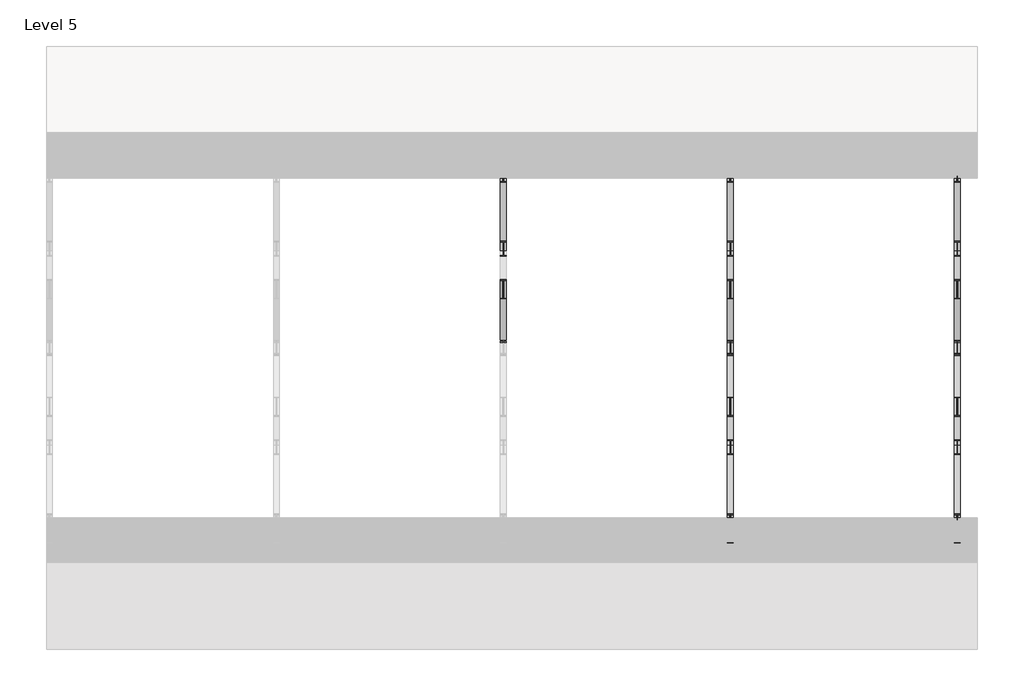
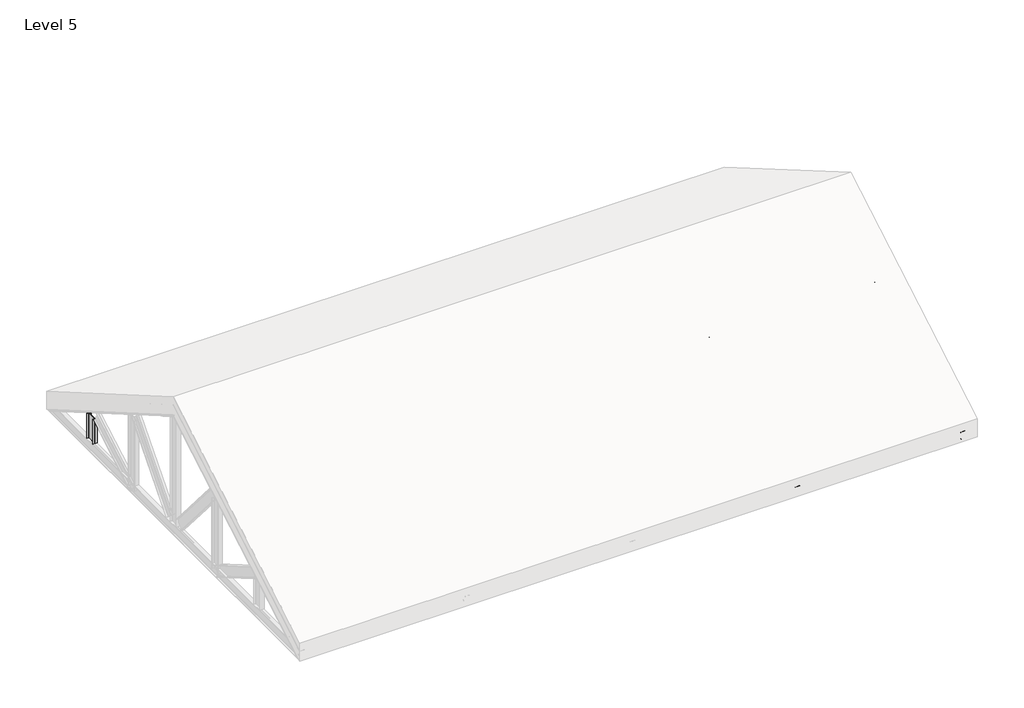
# One storey, part 2 of 2: 31 beams.
"""IFC4 building model written with IfcOpenShell, lengths in millimetres."""

from ifc_helpers import new_model, si_unit, frame, origin, place, context, project, spatial, polyline, circle_curve, ellipse_curve, transform, mapped, element, save
from ifc_brep_helpers import plane_surface, revolved_surface, advanced_brep
from components import ub_universal_beams_ub254x102x28_e74905dc, ub_universal_beams_ub254x102x28_1dca85a9, ub_universal_beams_ub254x102x28_3582687b, ub_universal_beams_ub254x102x28_9eef3cd1, ub_universal_beams_ub254x102x28_f7ef6108, ub_universal_beams_ub254x102x28_93a23aa5, ub_universal_beams_ub254x102x28_1ec9d6d8, ub_universal_beams_ub254x102x28_a06fb1b7

model = new_model("IFC4")

# Units and contexts
model_context = context("Model", 3, world=origin())
ifc_project = project(units=[si_unit("LENGTHUNIT", "METRE", prefix="MILLI")], contexts=[model_context])

# Site, building, storey
site = spatial("IfcSite", under=ifc_project)
building = spatial("IfcBuilding", under=site)
storey = spatial("IfcBuildingStorey", under=building, Name="Level 5", Elevation=9144.0)

# Beams
placement = place(None, origin())
element("IfcBeam", 1, ObjectType="UB-Universal Beams : UB254x102x28", at=placement, inside=storey, context=model_context, shape_type="AdvancedBrep", body=[
    advanced_brep(
    [(-879.5620752, 9795.4298445, 9040.0618528), (-879.5620752, 9790.4089662, 9031.4136864), (-981.7620752, 9790.4089662, 9031.4136864), (-981.7620752, 9795.4298445, 9040.0618528), (-941.4120752, 9795.4298445, 9040.0618528), (-933.8120752, 9799.245712, 9046.6344592), (-933.8120752, 9912.3158911, 9241.3911653), (-941.4120752, 9916.1317586, 9247.9637718), (-981.7620752, 9916.1317586, 9247.9637718), (-981.7620752, 9921.1526369, 9256.6119381), (-879.5620752, 9921.1526369, 9256.6119381), (-879.5620752, 9916.1317586, 9247.9637718), (-919.9120752, 9916.1317586, 9247.9637718), (-927.5120752, 9912.3158911, 9241.3911653), (-927.5120752, 9799.245712, 9046.6344592), (-919.9120752, 9795.4298445, 9040.0618528), (-919.9120752, 4605.8028699, 12053.0109991), (-879.5620752, 4605.8028699, 12053.0109991), (-927.5120752, 4605.8028699, 12061.7989892), (-927.5120752, 4605.8028699, 12322.2010108), (-919.9120752, 4605.8028699, 12330.9890009), (-879.5620752, 4605.8028699, 12330.9890009), (-879.5620752, 4605.8028699, 12342.5521457), (-981.7620752, 4605.8028699, 12342.5521457), (-981.7620752, 4605.8028699, 12330.9890009), (-941.4120752, 4605.8028699, 12330.9890009), (-933.8120752, 4605.8028699, 12322.2010108), (-933.8120752, 4605.8028699, 12061.7989892), (-941.4120752, 4605.8028699, 12053.0109991), (-981.7620752, 4605.8028699, 12053.0109991), (-981.7620752, 4605.8028699, 12041.4478543), (-879.5620752, 4605.8028699, 12041.4478543)],
    [
        (0, 1),
        (1, 2),
        (2, 3),
        (3, 4),
        (4, 5, circle_curve(frame((-941.4120752, 9799.245712, 9046.6344592), z_axis=(0.0, -0.8648166348106393, 0.5020878291243489), x_axis=(-1.0, 0.0, 0.0)), 7.6)),
        (5, 6),
        (6, 7, circle_curve(frame((-941.4120752, 9912.3158911, 9241.3911653), z_axis=(0.0, -0.8648166348106393, 0.5020878291243489), x_axis=(-1.0, 0.0, 0.0)), 7.6)),
        (7, 8),
        (8, 9),
        (9, 10),
        (10, 11),
        (11, 12),
        (12, 13, circle_curve(frame((-919.9120752, 9912.3158911, 9241.3911653), z_axis=(0.0, -0.8648166348106393, 0.5020878291243489), x_axis=(-1.0, 0.0, 0.0)), 7.6)),
        (13, 14),
        (14, 15, circle_curve(frame((-919.9120752, 9799.245712, 9046.6344592), z_axis=(0.0, -0.8648166348106393, 0.5020878291243489), x_axis=(-1.0, 0.0, 0.0)), 7.6)),
        (15, 0),
        (16, 17),
        (17, 0),
        (15, 16),
        (18, 16, ellipse_curve(frame((-919.9120752, 4605.8028699, 12061.7989892), z_axis=(0.0, -1.0, 0.0), x_axis=(0.0, 0.0, -1.0)), 8.7879901, 7.6)),
        (14, 18),
        (19, 18),
        (13, 19),
        (20, 19, ellipse_curve(frame((-919.9120752, 4605.8028699, 12322.2010108), z_axis=(0.0, -1.0, 0.0), x_axis=(0.0, 0.0, -1.0)), 8.7879901, 7.6)),
        (12, 20),
        (21, 20),
        (11, 21),
        (22, 21),
        (10, 22),
        (23, 22),
        (9, 23),
        (24, 23),
        (8, 24),
        (25, 24),
        (7, 25),
        (26, 25, ellipse_curve(frame((-941.4120752, 4605.8028699, 12322.2010108), z_axis=(0.0, -1.0, 0.0), x_axis=(0.0, 0.0, -1.0)), 8.7879901, 7.6)),
        (6, 26),
        (27, 26),
        (5, 27),
        (28, 27, ellipse_curve(frame((-941.4120752, 4605.8028699, 12061.7989892), z_axis=(0.0, -1.0, 0.0), x_axis=(0.0, 0.0, -1.0)), 8.7879901, 7.6)),
        (4, 28),
        (29, 28),
        (3, 29),
        (30, 29),
        (2, 30),
        (31, 30),
        (1, 31),
        (17, 31),
    ],
    [
        plane_surface(frame((-930.6620752, 9855.7808016, 9144.0128123), z_axis=(0.0, 0.8648166348106393, -0.5020878291243489), x_axis=(0.0, 0.5020878291243489, 0.8648166348106393))),
        plane_surface(frame((-879.5620752, 4545.4739812, 12088.0362282), z_axis=(0.0, 0.5020878291243489, 0.8648166348106393), x_axis=(0.0, 0.8648166348106393, -0.5020878291243489))),
        revolved_surface(polyline([(-927.5120752, 9799.245712003027, 9046.634459205212), (-927.5120752, 4601.987002407376, 12064.01437289046)]), (-919.9120752, 4549.2898487, 12094.6088347), (0.0, 0.8648166348106393, -0.5020878291243489)),
        plane_surface(frame((-927.5120752, 4549.2898487, 12094.6088347), z_axis=(1.0, 0.0, 0.0), x_axis=(0.0, 0.8648166348106393, -0.5020878291243489))),
        revolved_surface(polyline([(-927.5120752, 9912.315891103026, 9241.391165305211), (-927.5120752, 4601.987002367825, 12324.416394422336)]), (-919.9120752, 4662.3600278, 12289.3655408), (0.0, 0.8648166348106393, -0.5020878291243489)),
        plane_surface(frame((-919.9120752, 4666.1758953, 12295.9381472), z_axis=(0.0, -0.5020878291243489, -0.8648166348106393), x_axis=(0.0, 0.8648166348106393, -0.5020878291243489))),
        plane_surface(frame((-879.5620752, 4666.1758953, 12295.9381472), z_axis=(1.0, 0.0, 0.0), x_axis=(0.0, 0.8648166348106393, -0.5020878291243489))),
        plane_surface(frame((-879.5620752, 4671.1967736, 12304.5863136), z_axis=(0.0, 0.5020878291243489, 0.8648166348106393), x_axis=(0.0, 0.8648166348106393, -0.5020878291243489))),
        plane_surface(frame((-981.7620752, 4671.1967736, 12304.5863136), z_axis=(-1.0, 0.0, 0.0), x_axis=(0.0, 0.8648166348106393, -0.5020878291243489))),
        plane_surface(frame((-981.7620752, 4666.1758953, 12295.9381472), z_axis=(0.0, -0.5020878291243489, -0.8648166348106393), x_axis=(0.0, 0.8648166348106393, -0.5020878291243489))),
        revolved_surface(polyline([(-949.0120752, 9912.315891103026, 9241.391165305211), (-949.0120752, 4601.987002367825, 12324.416394422336)]), (-941.4120752, 4662.3600278, 12289.3655408), (0.0, 0.8648166348106393, -0.5020878291243489)),
        plane_surface(frame((-933.8120752, 4662.3600278, 12289.3655408), z_axis=(-1.0, 0.0, 0.0), x_axis=(0.0, 0.8648166348106393, -0.5020878291243489))),
        revolved_surface(polyline([(-949.0120752, 9799.245712003027, 9046.634459205212), (-949.0120752, 4601.987002407376, 12064.01437289046)]), (-941.4120752, 4549.2898487, 12094.6088347), (0.0, 0.8648166348106393, -0.5020878291243489)),
        plane_surface(frame((-941.4120752, 4545.4739812, 12088.0362282), z_axis=(0.0, 0.5020878291243489, 0.8648166348106393), x_axis=(0.0, 0.8648166348106393, -0.5020878291243489))),
        plane_surface(frame((-981.7620752, 4545.4739812, 12088.0362282), z_axis=(-1.0, 0.0, 0.0), x_axis=(0.0, 0.8648166348106393, -0.5020878291243489))),
        plane_surface(frame((-981.7620752, 4540.4531029, 12079.3880619), z_axis=(0.0, -0.5020878291243489, -0.8648166348106393), x_axis=(0.0, 0.8648166348106393, -0.5020878291243489))),
        plane_surface(frame((-879.5620752, 4540.4531029, 12079.3880619), z_axis=(1.0, 0.0, 0.0), x_axis=(0.0, 0.8648166348106393, -0.5020878291243489))),
        plane_surface(frame((-930.6620752, 4605.8028699, 12342.5521457), z_axis=(0.0, -1.0, 0.0), x_axis=(0.0, 0.0, 1.0))),
    ],
    [
        (0, [[1, 2, 3, 4, 5, 6, 7, 8, 9, 10, 11, 12, 13, 14, 15, 16]]),
        (1, [[17, 18, -16, 19]]),
        (2, [[20, -19, -15, 21]]),
        (3, [[22, -21, -14, 23]]),
        (4, [[24, -23, -13, 25]]),
        (5, [[26, -25, -12, 27]]),
        (6, [[28, -27, -11, 29]]),
        (7, [[30, -29, -10, 31]]),
        (8, [[32, -31, -9, 33]]),
        (9, [[34, -33, -8, 35]]),
        (10, [[36, -35, -7, 37]]),
        (11, [[38, -37, -6, 39]]),
        (12, [[40, -39, -5, 41]]),
        (13, [[42, -41, -4, 43]]),
        (14, [[44, -43, -3, 45]]),
        (15, [[46, -45, -2, 47]]),
        (16, [[48, -47, -1, -18]]),
        (17, [[-17, -20, -22, -24, -26, -28, -30, -32, -34, -36, -38, -40, -42, -44, -46, -48]]),
    ],
),
])
element("IfcBeam", 2, ObjectType="UB-Universal Beams : UB254x102x28", at=placement, inside=storey, context=model_context, shape_type="AdvancedBrep", body=[
    advanced_brep(
    [(3120.4379248, 9795.4298445, 9040.0618528), (3120.4379248, 9790.4089662, 9031.4136864), (3018.2379248, 9790.4089662, 9031.4136864), (3018.2379248, 9795.4298445, 9040.0618528), (3058.5879248, 9795.4298445, 9040.0618528), (3066.1879248, 9799.245712, 9046.6344592), (3066.1879248, 9912.3158911, 9241.3911653), (3058.5879248, 9916.1317586, 9247.9637718), (3018.2379248, 9916.1317586, 9247.9637718), (3018.2379248, 9921.1526369, 9256.6119381), (3120.4379248, 9921.1526369, 9256.6119381), (3120.4379248, 9916.1317586, 9247.9637718), (3080.0879248, 9916.1317586, 9247.9637718), (3072.4879248, 9912.3158911, 9241.3911653), (3072.4879248, 9799.245712, 9046.6344592), (3080.0879248, 9795.4298445, 9040.0618528), (3080.0879248, 4605.8028699, 12053.0109991), (3120.4379248, 4605.8028699, 12053.0109991), (3072.4879248, 4605.8028699, 12061.7989892), (3072.4879248, 4605.8028699, 12322.2010108), (3080.0879248, 4605.8028699, 12330.9890009), (3120.4379248, 4605.8028699, 12330.9890009), (3120.4379248, 4605.8028699, 12342.5521457), (3018.2379248, 4605.8028699, 12342.5521457), (3018.2379248, 4605.8028699, 12330.9890009), (3058.5879248, 4605.8028699, 12330.9890009), (3066.1879248, 4605.8028699, 12322.2010108), (3066.1879248, 4605.8028699, 12061.7989892), (3058.5879248, 4605.8028699, 12053.0109991), (3018.2379248, 4605.8028699, 12053.0109991), (3018.2379248, 4605.8028699, 12041.4478543), (3120.4379248, 4605.8028699, 12041.4478543)],
    [
        (0, 1),
        (1, 2),
        (2, 3),
        (3, 4),
        (4, 5, circle_curve(frame((3058.5879248, 9799.245712, 9046.6344592), z_axis=(0.0, -0.8648166348106393, 0.5020878291243489), x_axis=(-1.0, 0.0, 0.0)), 7.6)),
        (5, 6),
        (6, 7, circle_curve(frame((3058.5879248, 9912.3158911, 9241.3911653), z_axis=(0.0, -0.8648166348106393, 0.5020878291243489), x_axis=(-1.0, 0.0, 0.0)), 7.6)),
        (7, 8),
        (8, 9),
        (9, 10),
        (10, 11),
        (11, 12),
        (12, 13, circle_curve(frame((3080.0879248, 9912.3158911, 9241.3911653), z_axis=(0.0, -0.8648166348106393, 0.5020878291243489), x_axis=(-1.0, 0.0, 0.0)), 7.6)),
        (13, 14),
        (14, 15, circle_curve(frame((3080.0879248, 9799.245712, 9046.6344592), z_axis=(0.0, -0.8648166348106393, 0.5020878291243489), x_axis=(-1.0, 0.0, 0.0)), 7.6)),
        (15, 0),
        (16, 17),
        (17, 0),
        (15, 16),
        (18, 16, ellipse_curve(frame((3080.0879248, 4605.8028699, 12061.7989892), z_axis=(0.0, -1.0, 0.0), x_axis=(0.0, 0.0, -1.0)), 8.7879901, 7.6)),
        (14, 18),
        (19, 18),
        (13, 19),
        (20, 19, ellipse_curve(frame((3080.0879248, 4605.8028699, 12322.2010108), z_axis=(0.0, -1.0, 0.0), x_axis=(0.0, 0.0, -1.0)), 8.7879901, 7.6)),
        (12, 20),
        (21, 20),
        (11, 21),
        (22, 21),
        (10, 22),
        (23, 22),
        (9, 23),
        (24, 23),
        (8, 24),
        (25, 24),
        (7, 25),
        (26, 25, ellipse_curve(frame((3058.5879248, 4605.8028699, 12322.2010108), z_axis=(0.0, -1.0, 0.0), x_axis=(0.0, 0.0, -1.0)), 8.7879901, 7.6)),
        (6, 26),
        (27, 26),
        (5, 27),
        (28, 27, ellipse_curve(frame((3058.5879248, 4605.8028699, 12061.7989892), z_axis=(0.0, -1.0, 0.0), x_axis=(0.0, 0.0, -1.0)), 8.7879901, 7.6)),
        (4, 28),
        (29, 28),
        (3, 29),
        (30, 29),
        (2, 30),
        (31, 30),
        (1, 31),
        (17, 31),
    ],
    [
        plane_surface(frame((3069.3379248, 9855.7808016, 9144.0128123), z_axis=(0.0, 0.8648166348106393, -0.5020878291243489), x_axis=(0.0, 0.5020878291243489, 0.8648166348106393))),
        plane_surface(frame((3120.4379248, 4545.4739812, 12088.0362282), z_axis=(0.0, 0.5020878291243489, 0.8648166348106393), x_axis=(0.0, 0.8648166348106393, -0.5020878291243489))),
        revolved_surface(polyline([(3072.4879248, 9799.245712003027, 9046.634459205212), (3072.4879248, 4601.987002407376, 12064.01437289046)]), (3080.0879248, 4549.2898487, 12094.6088347), (0.0, 0.8648166348106393, -0.5020878291243489)),
        plane_surface(frame((3072.4879248, 4549.2898487, 12094.6088347), z_axis=(1.0, 0.0, 0.0), x_axis=(0.0, 0.8648166348106393, -0.5020878291243489))),
        revolved_surface(polyline([(3072.4879248, 9912.315891103026, 9241.391165305211), (3072.4879248, 4601.987002367825, 12324.416394422336)]), (3080.0879248, 4662.3600278, 12289.3655408), (0.0, 0.8648166348106393, -0.5020878291243489)),
        plane_surface(frame((3080.0879248, 4666.1758953, 12295.9381472), z_axis=(0.0, -0.5020878291243489, -0.8648166348106393), x_axis=(0.0, 0.8648166348106393, -0.5020878291243489))),
        plane_surface(frame((3120.4379248, 4666.1758953, 12295.9381472), z_axis=(1.0, 0.0, 0.0), x_axis=(0.0, 0.8648166348106393, -0.5020878291243489))),
        plane_surface(frame((3120.4379248, 4671.1967736, 12304.5863136), z_axis=(0.0, 0.5020878291243489, 0.8648166348106393), x_axis=(0.0, 0.8648166348106393, -0.5020878291243489))),
        plane_surface(frame((3018.2379248, 4671.1967736, 12304.5863136), z_axis=(-1.0, 0.0, 0.0), x_axis=(0.0, 0.8648166348106393, -0.5020878291243489))),
        plane_surface(frame((3018.2379248, 4666.1758953, 12295.9381472), z_axis=(0.0, -0.5020878291243489, -0.8648166348106393), x_axis=(0.0, 0.8648166348106393, -0.5020878291243489))),
        revolved_surface(polyline([(3050.9879248, 9912.315891103026, 9241.391165305211), (3050.9879248, 4601.987002367825, 12324.416394422336)]), (3058.5879248, 4662.3600278, 12289.3655408), (0.0, 0.8648166348106393, -0.5020878291243489)),
        plane_surface(frame((3066.1879248, 4662.3600278, 12289.3655408), z_axis=(-1.0, 0.0, 0.0), x_axis=(0.0, 0.8648166348106393, -0.5020878291243489))),
        revolved_surface(polyline([(3050.9879248, 9799.245712003027, 9046.634459205212), (3050.9879248, 4601.987002407376, 12064.01437289046)]), (3058.5879248, 4549.2898487, 12094.6088347), (0.0, 0.8648166348106393, -0.5020878291243489)),
        plane_surface(frame((3058.5879248, 4545.4739812, 12088.0362282), z_axis=(0.0, 0.5020878291243489, 0.8648166348106393), x_axis=(0.0, 0.8648166348106393, -0.5020878291243489))),
        plane_surface(frame((3018.2379248, 4545.4739812, 12088.0362282), z_axis=(-1.0, 0.0, 0.0), x_axis=(0.0, 0.8648166348106393, -0.5020878291243489))),
        plane_surface(frame((3018.2379248, 4540.4531029, 12079.3880619), z_axis=(0.0, -0.5020878291243489, -0.8648166348106393), x_axis=(0.0, 0.8648166348106393, -0.5020878291243489))),
        plane_surface(frame((3120.4379248, 4540.4531029, 12079.3880619), z_axis=(1.0, 0.0, 0.0), x_axis=(0.0, 0.8648166348106393, -0.5020878291243489))),
        plane_surface(frame((3069.3379248, 4605.8028699, 12342.5521457), z_axis=(0.0, -1.0, 0.0), x_axis=(0.0, 0.0, 1.0))),
    ],
    [
        (0, [[1, 2, 3, 4, 5, 6, 7, 8, 9, 10, 11, 12, 13, 14, 15, 16]]),
        (1, [[17, 18, -16, 19]]),
        (2, [[20, -19, -15, 21]]),
        (3, [[22, -21, -14, 23]]),
        (4, [[24, -23, -13, 25]]),
        (5, [[26, -25, -12, 27]]),
        (6, [[28, -27, -11, 29]]),
        (7, [[30, -29, -10, 31]]),
        (8, [[32, -31, -9, 33]]),
        (9, [[34, -33, -8, 35]]),
        (10, [[36, -35, -7, 37]]),
        (11, [[38, -37, -6, 39]]),
        (12, [[40, -39, -5, 41]]),
        (13, [[42, -41, -4, 43]]),
        (14, [[44, -43, -3, 45]]),
        (15, [[46, -45, -2, 47]]),
        (16, [[48, -47, -1, -18]]),
        (17, [[-17, -20, -22, -24, -26, -28, -30, -32, -34, -36, -38, -40, -42, -44, -46, -48]]),
    ],
),
])
element("IfcBeam", 3, ObjectType="UB-Universal Beams : UB254x102x28", at=placement, inside=storey, context=model_context, shape_type="AdvancedBrep", body=[
    advanced_brep(
    [(3120.4379248, -583.8241047, 9040.0618528), (3080.0879248, -583.8241047, 9040.0618528), (3072.4879248, -587.6399722, 9046.6344592), (3072.4879248, -700.7101513, 9241.3911653), (3080.0879248, -704.5260188, 9247.9637718), (3120.4379248, -704.5260188, 9247.9637718), (3120.4379248, -709.5468971, 9256.6119381), (3018.2379248, -709.5468971, 9256.6119381), (3018.2379248, -704.5260188, 9247.9637718), (3058.5879248, -704.5260188, 9247.9637718), (3066.1879248, -700.7101513, 9241.3911653), (3066.1879248, -587.6399722, 9046.6344592), (3058.5879248, -583.8241047, 9040.0618528), (3018.2379248, -583.8241047, 9040.0618528), (3018.2379248, -578.8032264, 9031.4136864), (3120.4379248, -578.8032264, 9031.4136864), (3120.4379248, 4605.8028699, 12053.0109991), (3080.0879248, 4605.8028699, 12053.0109991), (3072.4879248, 4605.8028699, 12061.7989892), (3072.4879248, 4605.8028699, 12322.2010108), (3080.0879248, 4605.8028699, 12330.9890009), (3120.4379248, 4605.8028699, 12330.9890009), (3120.4379248, 4605.8028699, 12342.5521457), (3018.2379248, 4605.8028699, 12342.5521457), (3018.2379248, 4605.8028699, 12330.9890009), (3058.5879248, 4605.8028699, 12330.9890009), (3066.1879248, 4605.8028699, 12322.2010108), (3066.1879248, 4605.8028699, 12061.7989892), (3058.5879248, 4605.8028699, 12053.0109991), (3018.2379248, 4605.8028699, 12053.0109991), (3018.2379248, 4605.8028699, 12041.4478543), (3120.4379248, 4605.8028699, 12041.4478543)],
    [
        (0, 1),
        (1, 2, circle_curve(frame((3080.0879248, -587.6399722, 9046.6344592), z_axis=(0.0, 0.8648166348106395, 0.5020878291243485), x_axis=(-1.0, 0.0, 0.0)), 7.6)),
        (2, 3),
        (3, 4, circle_curve(frame((3080.0879248, -700.7101513, 9241.3911653), z_axis=(0.0, 0.8648166348106395, 0.5020878291243485), x_axis=(-1.0, 0.0, 0.0)), 7.6)),
        (4, 5),
        (5, 6),
        (6, 7),
        (7, 8),
        (8, 9),
        (9, 10, circle_curve(frame((3058.5879248, -700.7101513, 9241.3911653), z_axis=(0.0, 0.8648166348106395, 0.5020878291243485), x_axis=(-1.0, 0.0, 0.0)), 7.6)),
        (10, 11),
        (11, 12, circle_curve(frame((3058.5879248, -587.6399722, 9046.6344592), z_axis=(0.0, 0.8648166348106395, 0.5020878291243485), x_axis=(-1.0, 0.0, 0.0)), 7.6)),
        (12, 13),
        (13, 14),
        (14, 15),
        (15, 0),
        (0, 16),
        (16, 17),
        (17, 1),
        (17, 18, ellipse_curve(frame((3080.0879248, 4605.8028699, 12061.7989892), z_axis=(0.0, 1.0, 0.0), x_axis=(0.0, 0.0, 1.0)), 8.7879901, 7.6)),
        (18, 2),
        (18, 19),
        (19, 3),
        (19, 20, ellipse_curve(frame((3080.0879248, 4605.8028699, 12322.2010108), z_axis=(0.0, 1.0, 0.0), x_axis=(0.0, 0.0, 1.0)), 8.7879901, 7.6)),
        (20, 4),
        (20, 21),
        (21, 5),
        (21, 22),
        (22, 6),
        (22, 23),
        (23, 7),
        (23, 24),
        (24, 8),
        (24, 25),
        (25, 9),
        (25, 26, ellipse_curve(frame((3058.5879248, 4605.8028699, 12322.2010108), z_axis=(0.0, 1.0, 0.0), x_axis=(0.0, 0.0, 1.0)), 8.7879901, 7.6)),
        (26, 10),
        (26, 27),
        (27, 11),
        (27, 28, ellipse_curve(frame((3058.5879248, 4605.8028699, 12061.7989892), z_axis=(0.0, 1.0, 0.0), x_axis=(0.0, 0.0, 1.0)), 8.7879901, 7.6)),
        (28, 12),
        (28, 29),
        (29, 13),
        (29, 30),
        (30, 14),
        (30, 31),
        (31, 15),
        (31, 16),
    ],
    [
        plane_surface(frame((3069.3379248, -644.1750617, 9144.0128123), z_axis=(0.0, -0.8648166348106395, -0.5020878291243485), x_axis=(0.0, -0.5020878291243485, 0.8648166348106395))),
        plane_surface(frame((3120.4379248, -583.8241047, 9040.0618528), z_axis=(0.0, -0.5020878291243485, 0.8648166348106395), x_axis=(0.0, 0.8648166348106395, 0.5020878291243485))),
        revolved_surface(polyline([(3072.4879248, 4609.618737395652, 12064.014372885247), (3072.4879248, -587.6399722, 9046.6344592)]), (3080.0879248, -587.6399722, 9046.6344592), (0.0, 0.8648166348106395, 0.5020878291243485)),
        plane_surface(frame((3072.4879248, -587.6399722, 9046.6344592), z_axis=(1.0, 0.0, 0.0), x_axis=(0.0, 0.8648166348106395, 0.5020878291243485))),
        revolved_surface(polyline([(3072.4879248, 4609.618737435201, 12324.416394417123), (3072.4879248, -700.7101513, 9241.3911653)]), (3080.0879248, -700.7101513, 9241.3911653), (0.0, 0.8648166348106395, 0.5020878291243485)),
        plane_surface(frame((3080.0879248, -704.5260188, 9247.9637718), z_axis=(0.0, 0.5020878291243485, -0.8648166348106395), x_axis=(0.0, 0.8648166348106395, 0.5020878291243485))),
        plane_surface(frame((3120.4379248, -704.5260188, 9247.9637718), z_axis=(1.0, 0.0, 0.0), x_axis=(0.0, 0.8648166348106395, 0.5020878291243485))),
        plane_surface(frame((3120.4379248, -709.5468971, 9256.6119381), z_axis=(0.0, -0.5020878291243485, 0.8648166348106395), x_axis=(0.0, 0.8648166348106395, 0.5020878291243485))),
        plane_surface(frame((3018.2379248, -709.5468971, 9256.6119381), z_axis=(-1.0, 0.0, 0.0), x_axis=(0.0, 0.8648166348106395, 0.5020878291243485))),
        plane_surface(frame((3018.2379248, -704.5260188, 9247.9637718), z_axis=(0.0, 0.5020878291243485, -0.8648166348106395), x_axis=(0.0, 0.8648166348106395, 0.5020878291243485))),
        revolved_surface(polyline([(3050.9879248, 4609.618737435201, 12324.416394417123), (3050.9879248, -700.7101513, 9241.3911653)]), (3058.5879248, -700.7101513, 9241.3911653), (0.0, 0.8648166348106395, 0.5020878291243485)),
        plane_surface(frame((3066.1879248, -700.7101513, 9241.3911653), z_axis=(-1.0, 0.0, 0.0), x_axis=(0.0, 0.8648166348106395, 0.5020878291243485))),
        revolved_surface(polyline([(3050.9879248, 4609.618737395652, 12064.014372885247), (3050.9879248, -587.6399722, 9046.6344592)]), (3058.5879248, -587.6399722, 9046.6344592), (0.0, 0.8648166348106395, 0.5020878291243485)),
        plane_surface(frame((3058.5879248, -583.8241047, 9040.0618528), z_axis=(0.0, -0.5020878291243485, 0.8648166348106395), x_axis=(0.0, 0.8648166348106395, 0.5020878291243485))),
        plane_surface(frame((3018.2379248, -583.8241047, 9040.0618528), z_axis=(-1.0, 0.0, 0.0), x_axis=(0.0, 0.8648166348106395, 0.5020878291243485))),
        plane_surface(frame((3018.2379248, -578.8032264, 9031.4136864), z_axis=(0.0, 0.5020878291243485, -0.8648166348106395), x_axis=(0.0, 0.8648166348106395, 0.5020878291243485))),
        plane_surface(frame((3120.4379248, -578.8032264, 9031.4136864), z_axis=(1.0, 0.0, 0.0), x_axis=(0.0, 0.8648166348106395, 0.5020878291243485))),
        plane_surface(frame((3069.3379248, 4605.8028699, 12342.5521457), z_axis=(0.0, 1.0, 0.0), x_axis=(0.0, 0.0, -1.0))),
    ],
    [
        (0, [[1, 2, 3, 4, 5, 6, 7, 8, 9, 10, 11, 12, 13, 14, 15, 16]]),
        (1, [[-1, 17, 18, 19]]),
        (2, [[-2, -19, 20, 21]]),
        (3, [[-3, -21, 22, 23]]),
        (4, [[-4, -23, 24, 25]]),
        (5, [[-5, -25, 26, 27]]),
        (6, [[-6, -27, 28, 29]]),
        (7, [[-7, -29, 30, 31]]),
        (8, [[-8, -31, 32, 33]]),
        (9, [[-9, -33, 34, 35]]),
        (10, [[-10, -35, 36, 37]]),
        (11, [[-11, -37, 38, 39]]),
        (12, [[-12, -39, 40, 41]]),
        (13, [[-13, -41, 42, 43]]),
        (14, [[-14, -43, 44, 45]]),
        (15, [[-15, -45, 46, 47]]),
        (16, [[-16, -47, 48, -17]]),
        (17, [[-48, -46, -44, -42, -40, -38, -36, -34, -32, -30, -28, -26, -24, -22, -20, -18]]),
    ],
),
])
element("IfcBeam", 4, ObjectType="UB-Universal Beams : UB254x102x28", at=placement, inside=storey, context=model_context, shape_type="AdvancedBrep", body=[
    advanced_brep(
    [(7120.4379248, 9795.4298445, 9040.0618528), (7120.4379248, 9790.4089662, 9031.4136864), (7018.2379248, 9790.4089662, 9031.4136864), (7018.2379248, 9795.4298445, 9040.0618528), (7058.5879248, 9795.4298445, 9040.0618528), (7066.1879248, 9799.245712, 9046.6344592), (7066.1879248, 9912.3158911, 9241.3911653), (7058.5879248, 9916.1317586, 9247.9637718), (7018.2379248, 9916.1317586, 9247.9637718), (7018.2379248, 9921.1526369, 9256.6119381), (7120.4379248, 9921.1526369, 9256.6119381), (7120.4379248, 9916.1317586, 9247.9637718), (7080.0879248, 9916.1317586, 9247.9637718), (7072.4879248, 9912.3158911, 9241.3911653), (7072.4879248, 9799.245712, 9046.6344592), (7080.0879248, 9795.4298445, 9040.0618528), (7080.0879248, 4605.8028699, 12053.0109991), (7120.4379248, 4605.8028699, 12053.0109991), (7072.4879248, 4605.8028699, 12061.7989892), (7072.4879248, 4605.8028699, 12322.2010108), (7080.0879248, 4605.8028699, 12330.9890009), (7120.4379248, 4605.8028699, 12330.9890009), (7120.4379248, 4605.8028699, 12342.5521457), (7018.2379248, 4605.8028699, 12342.5521457), (7018.2379248, 4605.8028699, 12330.9890009), (7058.5879248, 4605.8028699, 12330.9890009), (7066.1879248, 4605.8028699, 12322.2010108), (7066.1879248, 4605.8028699, 12061.7989892), (7058.5879248, 4605.8028699, 12053.0109991), (7018.2379248, 4605.8028699, 12053.0109991), (7018.2379248, 4605.8028699, 12041.4478543), (7120.4379248, 4605.8028699, 12041.4478543)],
    [
        (0, 1),
        (1, 2),
        (2, 3),
        (3, 4),
        (4, 5, circle_curve(frame((7058.5879248, 9799.245712, 9046.6344592), z_axis=(0.0, -0.8648166348106393, 0.5020878291243489), x_axis=(-1.0, 0.0, 0.0)), 7.6)),
        (5, 6),
        (6, 7, circle_curve(frame((7058.5879248, 9912.3158911, 9241.3911653), z_axis=(0.0, -0.8648166348106393, 0.5020878291243489), x_axis=(-1.0, 0.0, 0.0)), 7.6)),
        (7, 8),
        (8, 9),
        (9, 10),
        (10, 11),
        (11, 12),
        (12, 13, circle_curve(frame((7080.0879248, 9912.3158911, 9241.3911653), z_axis=(0.0, -0.8648166348106393, 0.5020878291243489), x_axis=(-1.0, 0.0, 0.0)), 7.6)),
        (13, 14),
        (14, 15, circle_curve(frame((7080.0879248, 9799.245712, 9046.6344592), z_axis=(0.0, -0.8648166348106393, 0.5020878291243489), x_axis=(-1.0, 0.0, 0.0)), 7.6)),
        (15, 0),
        (16, 17),
        (17, 0),
        (15, 16),
        (18, 16, ellipse_curve(frame((7080.0879248, 4605.8028699, 12061.7989892), z_axis=(0.0, -1.0, 0.0), x_axis=(0.0, 0.0, -1.0)), 8.7879901, 7.6)),
        (14, 18),
        (19, 18),
        (13, 19),
        (20, 19, ellipse_curve(frame((7080.0879248, 4605.8028699, 12322.2010108), z_axis=(0.0, -1.0, 0.0), x_axis=(0.0, 0.0, -1.0)), 8.7879901, 7.6)),
        (12, 20),
        (21, 20),
        (11, 21),
        (22, 21),
        (10, 22),
        (23, 22),
        (9, 23),
        (24, 23),
        (8, 24),
        (25, 24),
        (7, 25),
        (26, 25, ellipse_curve(frame((7058.5879248, 4605.8028699, 12322.2010108), z_axis=(0.0, -1.0, 0.0), x_axis=(0.0, 0.0, -1.0)), 8.7879901, 7.6)),
        (6, 26),
        (27, 26),
        (5, 27),
        (28, 27, ellipse_curve(frame((7058.5879248, 4605.8028699, 12061.7989892), z_axis=(0.0, -1.0, 0.0), x_axis=(0.0, 0.0, -1.0)), 8.7879901, 7.6)),
        (4, 28),
        (29, 28),
        (3, 29),
        (30, 29),
        (2, 30),
        (31, 30),
        (1, 31),
        (17, 31),
    ],
    [
        plane_surface(frame((7069.3379248, 9855.7808016, 9144.0128123), z_axis=(0.0, 0.8648166348106393, -0.5020878291243489), x_axis=(0.0, 0.5020878291243489, 0.8648166348106393))),
        plane_surface(frame((7120.4379248, 4545.4739812, 12088.0362282), z_axis=(0.0, 0.5020878291243489, 0.8648166348106393), x_axis=(0.0, 0.8648166348106393, -0.5020878291243489))),
        revolved_surface(polyline([(7072.4879248, 9799.245712003027, 9046.634459205212), (7072.4879248, 4601.987002407376, 12064.01437289046)]), (7080.0879248, 4549.2898487, 12094.6088347), (0.0, 0.8648166348106393, -0.5020878291243489)),
        plane_surface(frame((7072.4879248, 4549.2898487, 12094.6088347), z_axis=(1.0, 0.0, 0.0), x_axis=(0.0, 0.8648166348106393, -0.5020878291243489))),
        revolved_surface(polyline([(7072.4879248, 9912.315891103026, 9241.391165305211), (7072.4879248, 4601.987002367825, 12324.416394422336)]), (7080.0879248, 4662.3600278, 12289.3655408), (0.0, 0.8648166348106393, -0.5020878291243489)),
        plane_surface(frame((7080.0879248, 4666.1758953, 12295.9381472), z_axis=(0.0, -0.5020878291243489, -0.8648166348106393), x_axis=(0.0, 0.8648166348106393, -0.5020878291243489))),
        plane_surface(frame((7120.4379248, 4666.1758953, 12295.9381472), z_axis=(1.0, 0.0, 0.0), x_axis=(0.0, 0.8648166348106393, -0.5020878291243489))),
        plane_surface(frame((7120.4379248, 4671.1967736, 12304.5863136), z_axis=(0.0, 0.5020878291243489, 0.8648166348106393), x_axis=(0.0, 0.8648166348106393, -0.5020878291243489))),
        plane_surface(frame((7018.2379248, 4671.1967736, 12304.5863136), z_axis=(-1.0, 0.0, 0.0), x_axis=(0.0, 0.8648166348106393, -0.5020878291243489))),
        plane_surface(frame((7018.2379248, 4666.1758953, 12295.9381472), z_axis=(0.0, -0.5020878291243489, -0.8648166348106393), x_axis=(0.0, 0.8648166348106393, -0.5020878291243489))),
        revolved_surface(polyline([(7050.9879248, 9912.315891103026, 9241.391165305211), (7050.9879248, 4601.987002367825, 12324.416394422336)]), (7058.5879248, 4662.3600278, 12289.3655408), (0.0, 0.8648166348106393, -0.5020878291243489)),
        plane_surface(frame((7066.1879248, 4662.3600278, 12289.3655408), z_axis=(-1.0, 0.0, 0.0), x_axis=(0.0, 0.8648166348106393, -0.5020878291243489))),
        revolved_surface(polyline([(7050.9879248, 9799.245712003027, 9046.634459205212), (7050.9879248, 4601.987002407376, 12064.01437289046)]), (7058.5879248, 4549.2898487, 12094.6088347), (0.0, 0.8648166348106393, -0.5020878291243489)),
        plane_surface(frame((7058.5879248, 4545.4739812, 12088.0362282), z_axis=(0.0, 0.5020878291243489, 0.8648166348106393), x_axis=(0.0, 0.8648166348106393, -0.5020878291243489))),
        plane_surface(frame((7018.2379248, 4545.4739812, 12088.0362282), z_axis=(-1.0, 0.0, 0.0), x_axis=(0.0, 0.8648166348106393, -0.5020878291243489))),
        plane_surface(frame((7018.2379248, 4540.4531029, 12079.3880619), z_axis=(0.0, -0.5020878291243489, -0.8648166348106393), x_axis=(0.0, 0.8648166348106393, -0.5020878291243489))),
        plane_surface(frame((7120.4379248, 4540.4531029, 12079.3880619), z_axis=(1.0, 0.0, 0.0), x_axis=(0.0, 0.8648166348106393, -0.5020878291243489))),
        plane_surface(frame((7069.3379248, 4605.8028699, 12342.5521457), z_axis=(0.0, -1.0, 0.0), x_axis=(0.0, 0.0, 1.0))),
    ],
    [
        (0, [[1, 2, 3, 4, 5, 6, 7, 8, 9, 10, 11, 12, 13, 14, 15, 16]]),
        (1, [[17, 18, -16, 19]]),
        (2, [[20, -19, -15, 21]]),
        (3, [[22, -21, -14, 23]]),
        (4, [[24, -23, -13, 25]]),
        (5, [[26, -25, -12, 27]]),
        (6, [[28, -27, -11, 29]]),
        (7, [[30, -29, -10, 31]]),
        (8, [[32, -31, -9, 33]]),
        (9, [[34, -33, -8, 35]]),
        (10, [[36, -35, -7, 37]]),
        (11, [[38, -37, -6, 39]]),
        (12, [[40, -39, -5, 41]]),
        (13, [[42, -41, -4, 43]]),
        (14, [[44, -43, -3, 45]]),
        (15, [[46, -45, -2, 47]]),
        (16, [[48, -47, -1, -18]]),
        (17, [[-17, -20, -22, -24, -26, -28, -30, -32, -34, -36, -38, -40, -42, -44, -46, -48]]),
    ],
),
])
element("IfcBeam", 5, ObjectType="UB-Universal Beams : UB254x102x28", at=placement, inside=storey, context=model_context, shape_type="AdvancedBrep", body=[
    advanced_brep(
    [(7120.4379248, -583.8241047, 9040.0618528), (7080.0879248, -583.8241047, 9040.0618528), (7072.4879248, -587.6399722, 9046.6344592), (7072.4879248, -700.7101513, 9241.3911653), (7080.0879248, -704.5260188, 9247.9637718), (7120.4379248, -704.5260188, 9247.9637718), (7120.4379248, -709.5468971, 9256.6119381), (7018.2379248, -709.5468971, 9256.6119381), (7018.2379248, -704.5260188, 9247.9637718), (7058.5879248, -704.5260188, 9247.9637718), (7066.1879248, -700.7101513, 9241.3911653), (7066.1879248, -587.6399722, 9046.6344592), (7058.5879248, -583.8241047, 9040.0618528), (7018.2379248, -583.8241047, 9040.0618528), (7018.2379248, -578.8032264, 9031.4136864), (7120.4379248, -578.8032264, 9031.4136864), (7120.4379248, 4605.8028699, 12053.0109991), (7080.0879248, 4605.8028699, 12053.0109991), (7072.4879248, 4605.8028699, 12061.7989892), (7072.4879248, 4605.8028699, 12322.2010108), (7080.0879248, 4605.8028699, 12330.9890009), (7120.4379248, 4605.8028699, 12330.9890009), (7120.4379248, 4605.8028699, 12342.5521457), (7018.2379248, 4605.8028699, 12342.5521457), (7018.2379248, 4605.8028699, 12330.9890009), (7058.5879248, 4605.8028699, 12330.9890009), (7066.1879248, 4605.8028699, 12322.2010108), (7066.1879248, 4605.8028699, 12061.7989892), (7058.5879248, 4605.8028699, 12053.0109991), (7018.2379248, 4605.8028699, 12053.0109991), (7018.2379248, 4605.8028699, 12041.4478543), (7120.4379248, 4605.8028699, 12041.4478543)],
    [
        (0, 1),
        (1, 2, circle_curve(frame((7080.0879248, -587.6399722, 9046.6344592), z_axis=(0.0, 0.8648166348106395, 0.5020878291243485), x_axis=(-1.0, 0.0, 0.0)), 7.6)),
        (2, 3),
        (3, 4, circle_curve(frame((7080.0879248, -700.7101513, 9241.3911653), z_axis=(0.0, 0.8648166348106395, 0.5020878291243485), x_axis=(-1.0, 0.0, 0.0)), 7.6)),
        (4, 5),
        (5, 6),
        (6, 7),
        (7, 8),
        (8, 9),
        (9, 10, circle_curve(frame((7058.5879248, -700.7101513, 9241.3911653), z_axis=(0.0, 0.8648166348106395, 0.5020878291243485), x_axis=(-1.0, 0.0, 0.0)), 7.6)),
        (10, 11),
        (11, 12, circle_curve(frame((7058.5879248, -587.6399722, 9046.6344592), z_axis=(0.0, 0.8648166348106395, 0.5020878291243485), x_axis=(-1.0, 0.0, 0.0)), 7.6)),
        (12, 13),
        (13, 14),
        (14, 15),
        (15, 0),
        (0, 16),
        (16, 17),
        (17, 1),
        (17, 18, ellipse_curve(frame((7080.0879248, 4605.8028699, 12061.7989892), z_axis=(0.0, 1.0, 0.0), x_axis=(0.0, 0.0, 1.0)), 8.7879901, 7.6)),
        (18, 2),
        (18, 19),
        (19, 3),
        (19, 20, ellipse_curve(frame((7080.0879248, 4605.8028699, 12322.2010108), z_axis=(0.0, 1.0, 0.0), x_axis=(0.0, 0.0, 1.0)), 8.7879901, 7.6)),
        (20, 4),
        (20, 21),
        (21, 5),
        (21, 22),
        (22, 6),
        (22, 23),
        (23, 7),
        (23, 24),
        (24, 8),
        (24, 25),
        (25, 9),
        (25, 26, ellipse_curve(frame((7058.5879248, 4605.8028699, 12322.2010108), z_axis=(0.0, 1.0, 0.0), x_axis=(0.0, 0.0, 1.0)), 8.7879901, 7.6)),
        (26, 10),
        (26, 27),
        (27, 11),
        (27, 28, ellipse_curve(frame((7058.5879248, 4605.8028699, 12061.7989892), z_axis=(0.0, 1.0, 0.0), x_axis=(0.0, 0.0, 1.0)), 8.7879901, 7.6)),
        (28, 12),
        (28, 29),
        (29, 13),
        (29, 30),
        (30, 14),
        (30, 31),
        (31, 15),
        (31, 16),
    ],
    [
        plane_surface(frame((7069.3379248, -644.1750617, 9144.0128123), z_axis=(0.0, -0.8648166348106395, -0.5020878291243485), x_axis=(0.0, -0.5020878291243485, 0.8648166348106395))),
        plane_surface(frame((7120.4379248, -583.8241047, 9040.0618528), z_axis=(0.0, -0.5020878291243485, 0.8648166348106395), x_axis=(0.0, 0.8648166348106395, 0.5020878291243485))),
        revolved_surface(polyline([(7072.4879248, 4609.618737395652, 12064.014372885247), (7072.4879248, -587.6399722, 9046.6344592)]), (7080.0879248, -587.6399722, 9046.6344592), (0.0, 0.8648166348106395, 0.5020878291243485)),
        plane_surface(frame((7072.4879248, -587.6399722, 9046.6344592), z_axis=(1.0, 0.0, 0.0), x_axis=(0.0, 0.8648166348106395, 0.5020878291243485))),
        revolved_surface(polyline([(7072.4879248, 4609.618737435201, 12324.416394417123), (7072.4879248, -700.7101513, 9241.3911653)]), (7080.0879248, -700.7101513, 9241.3911653), (0.0, 0.8648166348106395, 0.5020878291243485)),
        plane_surface(frame((7080.0879248, -704.5260188, 9247.9637718), z_axis=(0.0, 0.5020878291243485, -0.8648166348106395), x_axis=(0.0, 0.8648166348106395, 0.5020878291243485))),
        plane_surface(frame((7120.4379248, -704.5260188, 9247.9637718), z_axis=(1.0, 0.0, 0.0), x_axis=(0.0, 0.8648166348106395, 0.5020878291243485))),
        plane_surface(frame((7120.4379248, -709.5468971, 9256.6119381), z_axis=(0.0, -0.5020878291243485, 0.8648166348106395), x_axis=(0.0, 0.8648166348106395, 0.5020878291243485))),
        plane_surface(frame((7018.2379248, -709.5468971, 9256.6119381), z_axis=(-1.0, 0.0, 0.0), x_axis=(0.0, 0.8648166348106395, 0.5020878291243485))),
        plane_surface(frame((7018.2379248, -704.5260188, 9247.9637718), z_axis=(0.0, 0.5020878291243485, -0.8648166348106395), x_axis=(0.0, 0.8648166348106395, 0.5020878291243485))),
        revolved_surface(polyline([(7050.9879248, 4609.618737435201, 12324.416394417123), (7050.9879248, -700.7101513, 9241.3911653)]), (7058.5879248, -700.7101513, 9241.3911653), (0.0, 0.8648166348106395, 0.5020878291243485)),
        plane_surface(frame((7066.1879248, -700.7101513, 9241.3911653), z_axis=(-1.0, 0.0, 0.0), x_axis=(0.0, 0.8648166348106395, 0.5020878291243485))),
        revolved_surface(polyline([(7050.9879248, 4609.618737395652, 12064.014372885247), (7050.9879248, -587.6399722, 9046.6344592)]), (7058.5879248, -587.6399722, 9046.6344592), (0.0, 0.8648166348106395, 0.5020878291243485)),
        plane_surface(frame((7058.5879248, -583.8241047, 9040.0618528), z_axis=(0.0, -0.5020878291243485, 0.8648166348106395), x_axis=(0.0, 0.8648166348106395, 0.5020878291243485))),
        plane_surface(frame((7018.2379248, -583.8241047, 9040.0618528), z_axis=(-1.0, 0.0, 0.0), x_axis=(0.0, 0.8648166348106395, 0.5020878291243485))),
        plane_surface(frame((7018.2379248, -578.8032264, 9031.4136864), z_axis=(0.0, 0.5020878291243485, -0.8648166348106395), x_axis=(0.0, 0.8648166348106395, 0.5020878291243485))),
        plane_surface(frame((7120.4379248, -578.8032264, 9031.4136864), z_axis=(1.0, 0.0, 0.0), x_axis=(0.0, 0.8648166348106395, 0.5020878291243485))),
        plane_surface(frame((7069.3379248, 4605.8028699, 12342.5521457), z_axis=(0.0, 1.0, 0.0), x_axis=(0.0, 0.0, -1.0))),
    ],
    [
        (0, [[1, 2, 3, 4, 5, 6, 7, 8, 9, 10, 11, 12, 13, 14, 15, 16]]),
        (1, [[-1, 17, 18, 19]]),
        (2, [[-2, -19, 20, 21]]),
        (3, [[-3, -21, 22, 23]]),
        (4, [[-4, -23, 24, 25]]),
        (5, [[-5, -25, 26, 27]]),
        (6, [[-6, -27, 28, 29]]),
        (7, [[-7, -29, 30, 31]]),
        (8, [[-8, -31, 32, 33]]),
        (9, [[-9, -33, 34, 35]]),
        (10, [[-10, -35, 36, 37]]),
        (11, [[-11, -37, 38, 39]]),
        (12, [[-12, -39, 40, 41]]),
        (13, [[-13, -41, 42, 43]]),
        (14, [[-14, -43, 44, 45]]),
        (15, [[-15, -45, 46, 47]]),
        (16, [[-16, -47, 48, -17]]),
        (17, [[-48, -46, -44, -42, -40, -38, -36, -34, -32, -30, -28, -26, -24, -22, -20, -18]]),
    ],
),
])
ub_universal_beams_ub254x102x28_shape = ub_universal_beams_ub254x102x28_e74905dc(model_context)
element("IfcBeam", 6, ObjectType="UB-Universal Beams : UB254x102x28", at=placement, inside=storey, context=model_context, shape_type="MappedRepresentation", body=[
    mapped(ub_universal_beams_ub254x102x28_shape, transform((3069.3379248, 4605.8028699, 9144.0), x_axis=(0.0, -1.0, 0.0), y_axis=(1.0, 0.0, 0.0), z_axis=(0.0, 0.0, 1.0))),
])
element("IfcBeam", 7, ObjectType="UB-Universal Beams : UB254x102x28", at=placement, inside=storey, context=model_context, shape_type="MappedRepresentation", body=[
    mapped(ub_universal_beams_ub254x102x28_shape, transform((7069.3379248, 4605.8028699, 9144.0), x_axis=(0.0, -1.0, 0.0), y_axis=(1.0, 0.0, 0.0), z_axis=(0.0, 0.0, 1.0))),
])
ub_universal_beams_ub254x102x28_2_shape = ub_universal_beams_ub254x102x28_1dca85a9(model_context)
element("IfcBeam", 8, ObjectType="UB-Universal Beams : UB254x102x28", at=placement, inside=storey, context=model_context, shape_type="MappedRepresentation", body=[
    mapped(ub_universal_beams_ub254x102x28_2_shape, transform((3069.3379248, 4605.8028699, 10668.0), x_axis=(0.0, 0.0, 1.0), y_axis=(-1.0, 0.0, 0.0), z_axis=(0.0, -1.0, 0.0))),
])
element("IfcBeam", 9, ObjectType="UB-Universal Beams : UB254x102x28", at=placement, inside=storey, context=model_context, shape_type="MappedRepresentation", body=[
    mapped(ub_universal_beams_ub254x102x28_2_shape, transform((7069.3379248, 4605.8028699, 10668.0), x_axis=(0.0, 0.0, 1.0), y_axis=(-1.0, 0.0, 0.0), z_axis=(0.0, -1.0, 0.0))),
])
ub_universal_beams_ub254x102x28_3_shape = ub_universal_beams_ub254x102x28_3582687b(model_context)
element("IfcBeam", 10, ObjectType="UB-Universal Beams : UB254x102x28", at=placement, inside=storey, context=model_context, shape_type="MappedRepresentation", body=[
    mapped(ub_universal_beams_ub254x102x28_3_shape, transform((-930.6620752, 6355.8028699, 10160.0), x_axis=(0.0, 0.0, 1.0), y_axis=(-1.0, 0.0, 0.0), z_axis=(0.0, -1.0, 0.0))),
])
element("IfcBeam", 11, ObjectType="UB-Universal Beams : UB254x102x28", at=placement, inside=storey, context=model_context, shape_type="MappedRepresentation", body=[
    mapped(ub_universal_beams_ub254x102x28_3_shape, transform((3069.3379248, 6355.8028699, 10160.0), x_axis=(0.0, 0.0, 1.0), y_axis=(-1.0, 0.0, 0.0), z_axis=(0.0, -1.0, 0.0))),
])
element("IfcBeam", 12, ObjectType="UB-Universal Beams : UB254x102x28", at=placement, inside=storey, context=model_context, shape_type="MappedRepresentation", body=[
    mapped(ub_universal_beams_ub254x102x28_3_shape, transform((3069.3379248, 2855.8028699, 10160.0), x_axis=(0.0, 0.0, 1.0), y_axis=(-1.0, 0.0, 0.0), z_axis=(0.0, -1.0, 0.0))),
])
element("IfcBeam", 13, ObjectType="UB-Universal Beams : UB254x102x28", at=placement, inside=storey, context=model_context, shape_type="MappedRepresentation", body=[
    mapped(ub_universal_beams_ub254x102x28_3_shape, transform((7069.3379248, 6355.8028699, 10160.0), x_axis=(0.0, 0.0, 1.0), y_axis=(-1.0, 0.0, 0.0), z_axis=(0.0, -1.0, 0.0))),
])
element("IfcBeam", 14, ObjectType="UB-Universal Beams : UB254x102x28", at=placement, inside=storey, context=model_context, shape_type="MappedRepresentation", body=[
    mapped(ub_universal_beams_ub254x102x28_3_shape, transform((7069.3379248, 2855.8028699, 10160.0), x_axis=(0.0, 0.0, 1.0), y_axis=(-1.0, 0.0, 0.0), z_axis=(0.0, -1.0, 0.0))),
])
ub_universal_beams_ub254x102x28_4_shape = ub_universal_beams_ub254x102x28_9eef3cd1(model_context)
element("IfcBeam", 15, ObjectType="UB-Universal Beams : UB254x102x28", at=placement, inside=storey, context=model_context, shape_type="MappedRepresentation", body=[
    mapped(ub_universal_beams_ub254x102x28_4_shape, transform((-8930.6620752, 8105.8028699, 9652.0), x_axis=(0.0, 0.0, 1.0), y_axis=(-1.0, 0.0, 0.0), z_axis=(0.0, -1.0, 0.0))),
])
element("IfcBeam", 16, ObjectType="UB-Universal Beams : UB254x102x28", at=placement, inside=storey, context=model_context, shape_type="MappedRepresentation", body=[
    mapped(ub_universal_beams_ub254x102x28_4_shape, transform((-4930.6620752, 8105.8028699, 9652.0), x_axis=(0.0, 0.0, 1.0), y_axis=(-1.0, 0.0, 0.0), z_axis=(0.0, -1.0, 0.0))),
])
element("IfcBeam", 17, ObjectType="UB-Universal Beams : UB254x102x28", at=placement, inside=storey, context=model_context, shape_type="MappedRepresentation", body=[
    mapped(ub_universal_beams_ub254x102x28_4_shape, transform((-930.6620752, 8105.8028699, 9652.0), x_axis=(0.0, 0.0, 1.0), y_axis=(-1.0, 0.0, 0.0), z_axis=(0.0, -1.0, 0.0))),
])
element("IfcBeam", 18, ObjectType="UB-Universal Beams : UB254x102x28", at=placement, inside=storey, context=model_context, shape_type="MappedRepresentation", body=[
    mapped(ub_universal_beams_ub254x102x28_4_shape, transform((3069.3379248, 8105.8028699, 9652.0), x_axis=(0.0, 0.0, 1.0), y_axis=(-1.0, 0.0, 0.0), z_axis=(0.0, -1.0, 0.0))),
])
element("IfcBeam", 19, ObjectType="UB-Universal Beams : UB254x102x28", at=placement, inside=storey, context=model_context, shape_type="MappedRepresentation", body=[
    mapped(ub_universal_beams_ub254x102x28_4_shape, transform((3069.3379248, 1105.8028699, 9652.0), x_axis=(0.0, 0.0, 1.0), y_axis=(-1.0, 0.0, 0.0), z_axis=(0.0, -1.0, 0.0))),
])
element("IfcBeam", 20, ObjectType="UB-Universal Beams : UB254x102x28", at=placement, inside=storey, context=model_context, shape_type="MappedRepresentation", body=[
    mapped(ub_universal_beams_ub254x102x28_4_shape, transform((7069.3379248, 8105.8028699, 9652.0), x_axis=(0.0, 0.0, 1.0), y_axis=(-1.0, 0.0, 0.0), z_axis=(0.0, -1.0, 0.0))),
])
element("IfcBeam", 21, ObjectType="UB-Universal Beams : UB254x102x28", at=placement, inside=storey, context=model_context, shape_type="MappedRepresentation", body=[
    mapped(ub_universal_beams_ub254x102x28_4_shape, transform((7069.3379248, 1105.8028699, 9652.0), x_axis=(0.0, 0.0, 1.0), y_axis=(-1.0, 0.0, 0.0), z_axis=(0.0, -1.0, 0.0))),
])
ub_universal_beams_ub254x102x28_5_shape = ub_universal_beams_ub254x102x28_f7ef6108(model_context)
element("IfcBeam", 22, ObjectType="UB-Universal Beams : UB254x102x28", at=placement, inside=storey, context=model_context, shape_type="MappedRepresentation", body=[
    mapped(ub_universal_beams_ub254x102x28_5_shape, transform((-930.6620752, 5480.8028699, 10160.0), x_axis=(0.0, -0.6525707169246113, -0.7577278267376082), y_axis=(-1.0, 0.0, 0.0), z_axis=(0.0, 0.7577278267376082, -0.6525707169246113))),
])
element("IfcBeam", 23, ObjectType="UB-Universal Beams : UB254x102x28", at=placement, inside=storey, context=model_context, shape_type="MappedRepresentation", body=[
    mapped(ub_universal_beams_ub254x102x28_5_shape, transform((3069.3379248, 5480.8028699, 10160.0), x_axis=(0.0, -0.6525707169246113, -0.7577278267376082), y_axis=(-1.0, 0.0, 0.0), z_axis=(0.0, 0.7577278267376082, -0.6525707169246113))),
])
element("IfcBeam", 24, ObjectType="UB-Universal Beams : UB254x102x28", at=placement, inside=storey, context=model_context, shape_type="MappedRepresentation", body=[
    mapped(ub_universal_beams_ub254x102x28_5_shape, transform((7069.3379248, 5480.8028699, 10160.0), x_axis=(0.0, -0.6525707169246113, -0.7577278267376082), y_axis=(-1.0, 0.0, 0.0), z_axis=(0.0, 0.7577278267376082, -0.6525707169246113))),
])
ub_universal_beams_ub254x102x28_6_shape = ub_universal_beams_ub254x102x28_93a23aa5(model_context)
element("IfcBeam", 25, ObjectType="UB-Universal Beams : UB254x102x28", at=placement, inside=storey, context=model_context, shape_type="MappedRepresentation", body=[
    mapped(ub_universal_beams_ub254x102x28_6_shape, transform((-930.6620752, 7230.8028699, 9652.0), x_axis=(0.0, -0.864816634810639, -0.5020878291243495), y_axis=(-1.0, 0.0, 0.0), z_axis=(0.0, 0.5020878291243495, -0.864816634810639))),
])
element("IfcBeam", 26, ObjectType="UB-Universal Beams : UB254x102x28", at=placement, inside=storey, context=model_context, shape_type="MappedRepresentation", body=[
    mapped(ub_universal_beams_ub254x102x28_6_shape, transform((3069.3379248, 7230.8028699, 9652.0), x_axis=(0.0, -0.864816634810639, -0.5020878291243495), y_axis=(-1.0, 0.0, 0.0), z_axis=(0.0, 0.5020878291243495, -0.864816634810639))),
])
element("IfcBeam", 27, ObjectType="UB-Universal Beams : UB254x102x28", at=placement, inside=storey, context=model_context, shape_type="MappedRepresentation", body=[
    mapped(ub_universal_beams_ub254x102x28_6_shape, transform((7069.3379248, 7230.8028699, 9652.0), x_axis=(0.0, -0.864816634810639, -0.5020878291243495), y_axis=(-1.0, 0.0, 0.0), z_axis=(0.0, 0.5020878291243495, -0.864816634810639))),
])
ub_universal_beams_ub254x102x28_7_shape = ub_universal_beams_ub254x102x28_1ec9d6d8(model_context)
element("IfcBeam", 28, ObjectType="UB-Universal Beams : UB254x102x28", at=placement, inside=storey, context=model_context, shape_type="MappedRepresentation", body=[
    mapped(ub_universal_beams_ub254x102x28_7_shape, transform((3069.3379248, 3730.8028699, 10160.0), x_axis=(0.0, -0.6525707169246112, 0.7577278267376083), y_axis=(-1.0, 0.0, 0.0), z_axis=(0.0, -0.7577278267376083, -0.6525707169246112))),
])
element("IfcBeam", 29, ObjectType="UB-Universal Beams : UB254x102x28", at=placement, inside=storey, context=model_context, shape_type="MappedRepresentation", body=[
    mapped(ub_universal_beams_ub254x102x28_7_shape, transform((7069.3379248, 3730.8028699, 10160.0), x_axis=(0.0, -0.6525707169246112, 0.7577278267376083), y_axis=(-1.0, 0.0, 0.0), z_axis=(0.0, -0.7577278267376083, -0.6525707169246112))),
])
ub_universal_beams_ub254x102x28_8_shape = ub_universal_beams_ub254x102x28_a06fb1b7(model_context)
element("IfcBeam", 30, ObjectType="UB-Universal Beams : UB254x102x28", at=placement, inside=storey, context=model_context, shape_type="MappedRepresentation", body=[
    mapped(ub_universal_beams_ub254x102x28_8_shape, transform((3069.3379248, 1980.8028699, 9652.0), x_axis=(0.0, -0.8648166348106384, 0.5020878291243502), y_axis=(-1.0, 0.0, 0.0), z_axis=(0.0, -0.5020878291243502, -0.8648166348106384))),
])
element("IfcBeam", 31, ObjectType="UB-Universal Beams : UB254x102x28", at=placement, inside=storey, context=model_context, shape_type="MappedRepresentation", body=[
    mapped(ub_universal_beams_ub254x102x28_8_shape, transform((7069.3379248, 1980.8028699, 9652.0), x_axis=(0.0, -0.8648166348106384, 0.5020878291243502), y_axis=(-1.0, 0.0, 0.0), z_axis=(0.0, -0.5020878291243502, -0.8648166348106384))),
])

save(model, "model.ifc")

# Revit data of these elements
# Type "UB-Universal Beams : UB254x102x28"
#   Section Name Key = "UB254X102X28"
#   Width = 10.22 cm
#   Web Thickness = 0.63 cm
#   Web Fillet = 0.76 cm
#   Warping Constant = 28000.0 cm⁶
#   Torsional Moment of Inertia = 9.57 cm⁴
#   Section Area = 36.1 cm²
#   Plastic Modulus weak axis = 54.8 cm³
#   Plastic Modulus strong axis = 353.0 cm³
#   Nominal Weight = 28.2999 kgf/m
#   Moment of Inertia weak axis = 179.00 cm⁴
#   Moment of Inertia strong axis = 4005.00 cm⁴
#   Height = 26.04 cm
#   Flange Thickness = 1.0 cm
#   Elastic Modulus weak axis = 34.9 cm³
#   Elastic Modulus strong axis = 308.0 cm³
#   Centroid Vertical = 13.02 cm
#   Centroid Horizontal = 5.11 cm
#   Bolt Spacing = 5.4 cm
#   Length [instance default] = 4' - 11.05512"
#   Structural Material [instance default] = Metal - Steel 43-275
#   Type Comments = ""
#   Assembly Code = ""
# Elements 1, 2, 3, 4, 5, 6, 7, 8, 9, 10, 11, 12, 13, 14, 15, 16, 17, 18, 19, 20, 21, 22, 23, 24, 25, 26, 27, 28, 29, 30, 31 (IfcBeam, "UB-Universal Beams : UB254x102x28")
#   Structural Material = Metal - Steel 43-275
#   Phase Created = New Construction
#   Materials on its faces: "Metal - Steel 43-275"
# Materials
#   "Metal - Steel 43-275": class "Metal", colour RGB 247 247 247, transparency 0, Cost = 0
